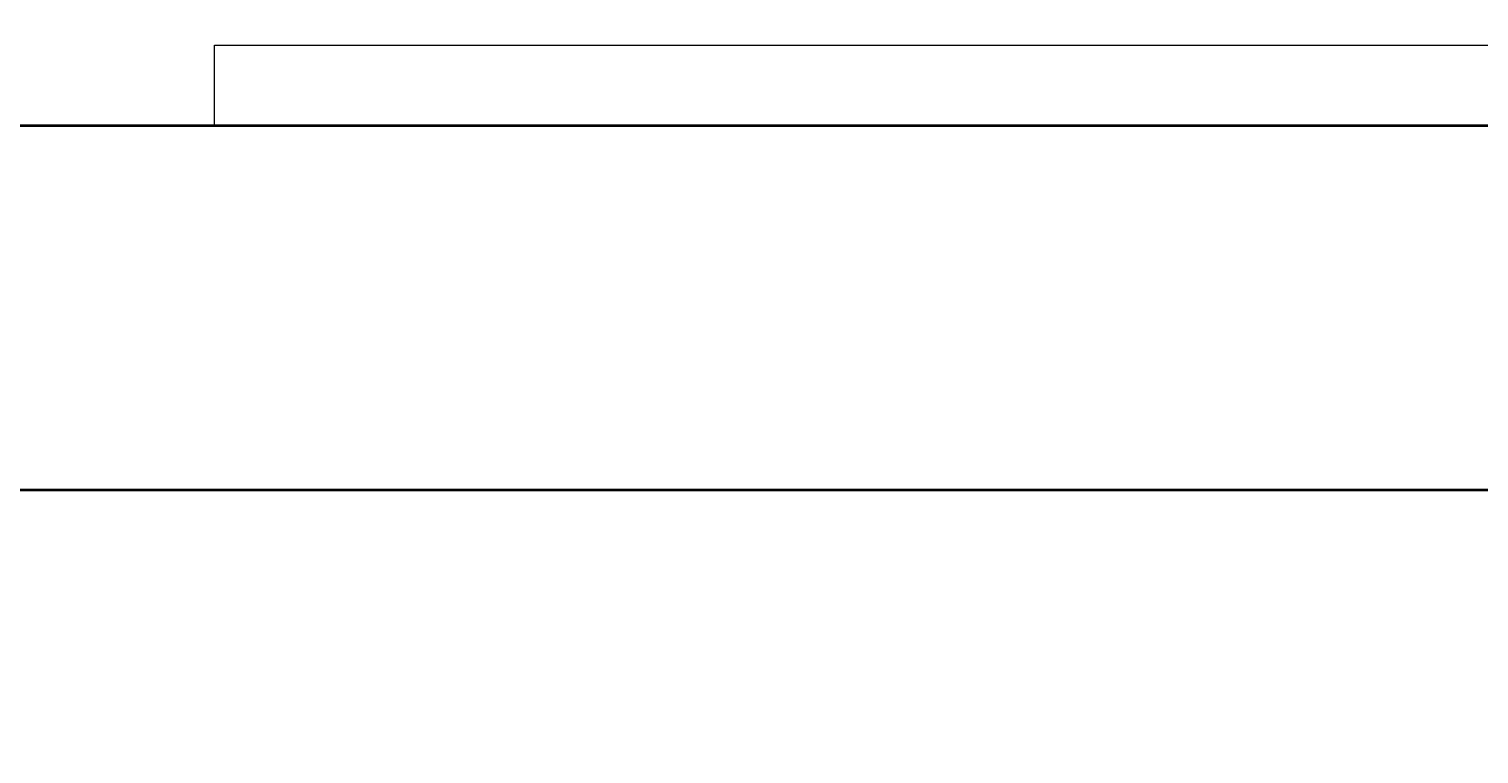
# Model space of a CAD drawing. Units: millimetres. Extents: x 27017497 to 27018854, y 7058029 to 7059154.
# Tile 67 of 91: x 27018355 to 27018390, y 7058126 to 7058144. Entities that reach past the tile are written whole.
import ezdxf

# ---------------------------------------------------------------- set-up
doc = ezdxf.new("R2010")
doc.units = ezdxf.units.MM
for name, color, linetype, lineweight in [('A-ANNO-DIMS', 2, 'Continuous', 18), ('A-FLOR-CASE-PATT', 44, 'Continuous', 13), ('A-FURN', 8, 'Continuous', 18), ('A-WALL', 7, 'Continuous', 35)]:
    doc.layers.add(name, color=color, linetype=linetype, lineweight=lineweight)
doc.styles.get("Standard").update_dxf_attribs({"font": 'arial.ttf'})
doc.dimstyles.get("Standard").update_dxf_attribs({"dimtxt": 0.18, "dimasz": 0.18, "dimexe": 0.18, "dimexo": 0.0625, "dimgap": 0.09, "dimtad": 0, "dimtih": 1, "dimtoh": 1, "dimdec": 4, "dimzin": 0, "dimdsep": 46, "dimtxsty": 'Standard', "dimcen": 0.09, "dimadec": 0, "dimazin": 0, "dimtfac": 1, "dimtdec": 4, "dimtofl": 0, "dimtmove": 0, "dimatfit": 3, "dimfxl": 1, "dimtolj": 1, "dimtzin": 0, "dimarcsym": 0})

# ---------------------------------------------------------------- blocks, each defined once
blk = doc.blocks.new('CAMMAT')
for p, q in [((1.27313, 0), (-1.27313, 0)), ((1.27313, 0), (1.27313, -0.05)), ((1.27313, -0.05), (-1.27313, -0.05))]:
    blk.add_line(p, q)
blk = doc.blocks.new('*D47')
at = {"layer": 'A-ANNO-DIMS', "color": 0, "lineweight": -2, "transparency": 16777216}
for p, q in [((27017561.166, 7058294.35), (27017561.166, 7058028.6)), ((27018790.606, 7058294.35), (27018790.606, 7058028.6)), ((27017561.346, 7058028.78), (27018175.431, 7058028.78)), ((27018790.426, 7058028.78), (27018176.341, 7058028.78))]:
    blk.add_line(p, q, dxfattribs=at)
at = {"layer": 'A-ANNO-DIMS', "color": 0, "transparency": 16777216}
for points in [[(27017561.346, 7058028.81), (27017561.346, 7058028.75), (27017561.166, 7058028.78)], [(27018790.426, 7058028.81), (27018790.426, 7058028.75), (27018790.606, 7058028.78)]]:
    blk.add_solid(points, dxfattribs=at)
at = {"layer": 'Defpoints', "color": 0, "transparency": 16777216}
for p in [(27017561.166, 7058294.412), (27018790.606, 7058294.412), (27018790.606, 7058028.78)]:
    blk.add_point(p, dxfattribs=at)
at = {"layer": 'A-ANNO-DIMS', "color": 0, "transparency": 16777216, "insert": (27018175.886, 7058028.78), "char_height": 0.18, "attachment_point": 5}
blk.add_mtext('\\A1;1229.4', dxfattribs=at)
blk = doc.blocks.new('*D48')
at = {"layer": 'A-ANNO-DIMS', "color": 0, "lineweight": -2, "transparency": 16777216}
for p, q in [((27018463.498, 7058622.912), (27017497.536, 7058622.912)), ((27017497.716, 7058622.732), (27017497.716, 7058357.753)), ((27017497.716, 7058092.41), (27017497.716, 7058357.389)), ((27018555.129, 7058092.23), (27017497.536, 7058092.23))]:
    blk.add_line(p, q, dxfattribs=at)
at = {"layer": 'A-ANNO-DIMS', "color": 0, "transparency": 16777216}
for points in [[(27017497.686, 7058622.732), (27017497.746, 7058622.732), (27017497.716, 7058622.912)], [(27017497.686, 7058092.41), (27017497.746, 7058092.41), (27017497.716, 7058092.23)]]:
    blk.add_solid(points, dxfattribs=at)
at = {"layer": 'Defpoints', "color": 0, "transparency": 16777216}
for p in [(27018463.561, 7058622.912), (27017497.716, 7058092.23), (27018555.192, 7058092.23)]:
    blk.add_point(p, dxfattribs=at)
at = {"layer": 'A-ANNO-DIMS', "color": 0, "transparency": 16777216, "insert": (27017497.716, 7058357.571), "char_height": 0.18, "attachment_point": 5}
blk.add_mtext('\\A1;530.7', dxfattribs=at)

msp = doc.modelspace()

# ---------------------------------------------------------------- hatches: boundary and pattern name
at = {"layer": 'A-FLOR-CASE-PATT'}
h = msp.add_hatch(color=256, dxfattribs=at)
h.dxf.hatch_style = 1
edge = h.paths.add_edge_path()
edge.add_line((27018341.343, 7058207.055), (27018330.837, 7058207.055))
edge.add_line((27018330.837, 7058207.055), (27018330.837, 7058203.02))
edge.add_line((27018330.837, 7058203.02), (27018338.424, 7058203.02))
edge.add_ellipse((27018338.23, 7058202.551), major_axis=(0.528, 0), ratio=0.888892, start_angle=0, end_angle=90, ccw=False)
edge.add_line((27018338.758, 7058202.551), (27018338.758, 7058202.238))
edge.add_line((27018338.758, 7058202.238), (27018330.837, 7058201.488))
edge.add_line((27018330.837, 7058201.488), (27018330.837, 7058199.747))
edge.add_line((27018330.837, 7058199.747), (27018338.424, 7058199.747))
edge.add_ellipse((27018338.23, 7058199.277), major_axis=(0.528, 0), ratio=0.888892, start_angle=0, end_angle=90, ccw=False)
edge.add_line((27018338.758, 7058199.277), (27018338.758, 7058198.964))
edge.add_line((27018338.758, 7058198.964), (27018330.837, 7058198.215))
edge.add_line((27018330.837, 7058198.215), (27018330.837, 7058193.415))
edge.add_line((27018330.837, 7058193.415), (27018338.284, 7058190.704))
edge.add_ellipse((27018337.942, 7058190.329), major_axis=(0.496, -0.181), ratio=0.888892, start_angle=0, end_angle=90, ccw=False)
edge.add_line((27018338.439, 7058190.148), (27018338.331, 7058189.854))
edge.add_line((27018338.331, 7058189.854), (27018330.837, 7058191.806))
edge.add_line((27018330.837, 7058191.806), (27018330.837, 7058188.22))
edge.add_line((27018330.837, 7058188.22), (27018338.424, 7058188.22))
edge.add_ellipse((27018338.23, 7058187.75), major_axis=(0.528, 0), ratio=0.888892, start_angle=0, end_angle=90, ccw=False)
edge.add_line((27018338.758, 7058187.75), (27018338.758, 7058187.437))
edge.add_line((27018338.758, 7058187.437), (27018330.837, 7058186.688))
edge.add_line((27018330.837, 7058186.688), (27018330.837, 7058181.982))
edge.add_line((27018330.837, 7058181.982), (27018338.424, 7058181.982))
edge.add_ellipse((27018338.23, 7058181.513), major_axis=(0.528, 0), ratio=0.888892, start_angle=0, end_angle=90, ccw=False)
edge.add_line((27018338.758, 7058181.513), (27018338.758, 7058181.199))
edge.add_line((27018338.758, 7058181.199), (27018330.837, 7058180.45))
edge.add_line((27018330.837, 7058180.45), (27018330.837, 7058178.709))
edge.add_line((27018330.837, 7058178.709), (27018338.424, 7058178.709))
edge.add_ellipse((27018338.23, 7058178.239), major_axis=(0.528, 0), ratio=0.888892, start_angle=0, end_angle=90, ccw=False)
edge.add_line((27018338.758, 7058178.239), (27018338.758, 7058177.926))
edge.add_line((27018338.758, 7058177.926), (27018330.837, 7058177.177))
edge.add_line((27018330.837, 7058177.177), (27018330.837, 7058173.878))
edge.add_line((27018330.837, 7058173.878), (27018338.284, 7058171.167))
edge.add_ellipse((27018337.942, 7058170.792), major_axis=(0.496, -0.181), ratio=0.888892, start_angle=0, end_angle=90, ccw=False)
edge.add_line((27018338.439, 7058170.611), (27018338.331, 7058170.317))
edge.add_line((27018338.331, 7058170.317), (27018330.837, 7058172.269))
edge.add_line((27018330.837, 7058172.269), (27018330.837, 7058168.293))
edge.add_line((27018330.837, 7058168.293), (27018338.424, 7058168.293))
edge.add_ellipse((27018338.23, 7058167.824), major_axis=(0.528, 0), ratio=0.888892, start_angle=0, end_angle=90, ccw=False)
edge.add_line((27018338.758, 7058167.824), (27018338.758, 7058167.511))
edge.add_line((27018338.758, 7058167.511), (27018330.837, 7058166.762))
edge.add_line((27018330.837, 7058166.762), (27018330.837, 7058160.389))
edge.add_line((27018330.837, 7058160.389), (27018338.424, 7058160.389))
edge.add_ellipse((27018338.23, 7058159.92), major_axis=(0.528, 0), ratio=0.888892, start_angle=0, end_angle=90, ccw=False)
edge.add_line((27018338.758, 7058159.92), (27018338.758, 7058159.607))
edge.add_line((27018338.758, 7058159.607), (27018330.837, 7058158.858))
edge.add_line((27018330.837, 7058158.858), (27018330.837, 7058157.116))
edge.add_line((27018330.837, 7058157.116), (27018338.424, 7058157.116))
edge.add_ellipse((27018338.23, 7058156.647), major_axis=(0.528, 0), ratio=0.888892, start_angle=0, end_angle=90, ccw=False)
edge.add_line((27018338.758, 7058156.647), (27018338.758, 7058156.334))
edge.add_line((27018338.758, 7058156.334), (27018330.837, 7058155.585))
edge.add_line((27018330.837, 7058155.585), (27018330.837, 7058150.784))
edge.add_line((27018330.837, 7058150.784), (27018338.284, 7058148.073))
edge.add_ellipse((27018337.942, 7058147.698), major_axis=(0.496, -0.181), ratio=0.888892, start_angle=0, end_angle=90, ccw=False)
edge.add_line((27018338.439, 7058147.517), (27018338.331, 7058147.223))
edge.add_line((27018338.331, 7058147.223), (27018330.837, 7058149.175))
edge.add_line((27018330.837, 7058149.175), (27018330.837, 7058145.589))
edge.add_line((27018330.837, 7058145.589), (27018338.424, 7058145.589))
edge.add_ellipse((27018338.23, 7058145.119), major_axis=(0.528, 0), ratio=0.888892, start_angle=0, end_angle=90, ccw=False)
edge.add_line((27018338.758, 7058145.119), (27018338.758, 7058144.806))
edge.add_line((27018338.758, 7058144.806), (27018330.837, 7058144.057))
edge.add_line((27018330.837, 7058144.057), (27018330.837, 7058141.912))
edge.add_line((27018330.837, 7058141.912), (27018341.343, 7058141.912))
edge.add_line((27018341.343, 7058141.912), (27018341.343, 7058207.055))
edge = h.paths.add_edge_path()
edge.add_line((27018330.112, 7058207.055), (27018319.606, 7058207.055))
edge.add_line((27018319.606, 7058207.055), (27018319.606, 7058141.912))
edge.add_line((27018319.606, 7058141.912), (27018330.112, 7058141.912))
edge.add_line((27018330.112, 7058141.912), (27018330.112, 7058144.024))
edge.add_line((27018330.112, 7058144.024), (27018322.543, 7058144.024))
edge.add_ellipse((27018322.736, 7058144.493), major_axis=(0.528, 0), ratio=0.888892, start_angle=180, end_angle=270, ccw=False)
edge.add_line((27018322.208, 7058144.493), (27018322.208, 7058145.291))
edge.add_ellipse((27018322.736, 7058145.119), major_axis=(0.528, 0), ratio=0.888892, start_angle=90, end_angle=180, ccw=False)
edge.add_line((27018322.736, 7058145.589), (27018330.112, 7058145.589))
edge.add_line((27018330.112, 7058145.589), (27018330.112, 7058149.382))
edge.add_line((27018330.112, 7058149.382), (27018322.826, 7058152.034))
edge.add_ellipse((27018323.168, 7058152.409), major_axis=(0.496, -0.181), ratio=0.888892, start_angle=180, end_angle=270, ccw=False)
edge.add_line((27018322.672, 7058152.59), (27018322.945, 7058153.34))
edge.add_ellipse((27018323.382, 7058152.997), major_axis=(0.496, -0.181), ratio=0.888892, start_angle=90, end_angle=180, ccw=False)
edge.add_line((27018323.543, 7058153.439), (27018330.112, 7058151.048))
edge.add_line((27018330.112, 7058151.048), (27018330.112, 7058155.551))
edge.add_line((27018330.112, 7058155.551), (27018322.543, 7058155.551))
edge.add_ellipse((27018322.736, 7058156.021), major_axis=(0.528, 0), ratio=0.888892, start_angle=180, end_angle=270, ccw=False)
edge.add_line((27018322.208, 7058156.021), (27018322.208, 7058156.819))
edge.add_ellipse((27018322.736, 7058156.647), major_axis=(0.528, 0), ratio=0.888892, start_angle=90, end_angle=180, ccw=False)
edge.add_line((27018322.736, 7058157.116), (27018330.112, 7058157.116))
edge.add_line((27018330.112, 7058157.116), (27018330.112, 7058158.824))
edge.add_line((27018330.112, 7058158.824), (27018322.543, 7058158.824))
edge.add_ellipse((27018322.736, 7058159.294), major_axis=(0.528, 0), ratio=0.888892, start_angle=180, end_angle=270, ccw=False)
edge.add_line((27018322.208, 7058159.294), (27018322.208, 7058160.092))
edge.add_ellipse((27018322.736, 7058159.92), major_axis=(0.528, 0), ratio=0.888892, start_angle=90, end_angle=180, ccw=False)
edge.add_line((27018322.736, 7058160.389), (27018330.112, 7058160.389))
edge.add_line((27018330.112, 7058160.389), (27018330.112, 7058166.728))
edge.add_line((27018330.112, 7058166.728), (27018322.543, 7058166.728))
edge.add_ellipse((27018322.736, 7058167.198), major_axis=(0.528, 0), ratio=0.888892, start_angle=180, end_angle=270, ccw=False)
edge.add_line((27018322.208, 7058167.198), (27018322.208, 7058167.996))
edge.add_ellipse((27018322.736, 7058167.824), major_axis=(0.528, 0), ratio=0.888892, start_angle=90, end_angle=180, ccw=False)
edge.add_line((27018322.736, 7058168.293), (27018330.112, 7058168.293))
edge.add_line((27018330.112, 7058168.293), (27018330.112, 7058172.476))
edge.add_line((27018330.112, 7058172.476), (27018322.826, 7058175.128))
edge.add_ellipse((27018323.168, 7058175.503), major_axis=(0.496, -0.181), ratio=0.888892, start_angle=180, end_angle=270, ccw=False)
edge.add_line((27018322.672, 7058175.684), (27018322.945, 7058176.433))
edge.add_ellipse((27018323.382, 7058176.091), major_axis=(0.496, -0.181), ratio=0.888892, start_angle=90, end_angle=180, ccw=False)
edge.add_line((27018323.543, 7058176.533), (27018330.112, 7058174.142))
edge.add_line((27018330.112, 7058174.142), (27018330.112, 7058177.144))
edge.add_line((27018330.112, 7058177.144), (27018322.543, 7058177.144))
edge.add_ellipse((27018322.736, 7058177.613), major_axis=(0.528, 0), ratio=0.888892, start_angle=180, end_angle=270, ccw=False)
edge.add_line((27018322.208, 7058177.613), (27018322.208, 7058178.411))
edge.add_ellipse((27018322.736, 7058178.239), major_axis=(0.528, 0), ratio=0.888892, start_angle=90, end_angle=180, ccw=False)
edge.add_line((27018322.736, 7058178.709), (27018330.112, 7058178.709))
edge.add_line((27018330.112, 7058178.709), (27018330.112, 7058180.417))
edge.add_line((27018330.112, 7058180.417), (27018322.543, 7058180.417))
edge.add_ellipse((27018322.736, 7058180.886), major_axis=(0.528, 0), ratio=0.888892, start_angle=180, end_angle=270, ccw=False)
edge.add_line((27018322.208, 7058180.886), (27018322.208, 7058181.684))
edge.add_ellipse((27018322.736, 7058181.513), major_axis=(0.528, 0), ratio=0.888892, start_angle=90, end_angle=180, ccw=False)
edge.add_line((27018322.736, 7058181.982), (27018330.112, 7058181.982))
edge.add_line((27018330.112, 7058181.982), (27018330.112, 7058186.655))
edge.add_line((27018330.112, 7058186.655), (27018322.543, 7058186.655))
edge.add_ellipse((27018322.736, 7058187.124), major_axis=(0.528, 0), ratio=0.888892, start_angle=180, end_angle=270, ccw=False)
edge.add_line((27018322.208, 7058187.124), (27018322.208, 7058187.922))
edge.add_ellipse((27018322.736, 7058187.75), major_axis=(0.528, 0), ratio=0.888892, start_angle=90, end_angle=180, ccw=False)
edge.add_line((27018322.736, 7058188.22), (27018330.112, 7058188.22))
edge.add_line((27018330.112, 7058188.22), (27018330.112, 7058192.013))
edge.add_line((27018330.112, 7058192.013), (27018322.826, 7058194.665))
edge.add_ellipse((27018323.168, 7058195.04), major_axis=(0.496, -0.181), ratio=0.888892, start_angle=180, end_angle=270, ccw=False)
edge.add_line((27018322.672, 7058195.22), (27018322.945, 7058195.97))
edge.add_ellipse((27018323.382, 7058195.628), major_axis=(0.496, -0.181), ratio=0.888892, start_angle=90, end_angle=180, ccw=False)
edge.add_line((27018323.543, 7058196.069), (27018330.112, 7058193.678))
edge.add_line((27018330.112, 7058193.678), (27018330.112, 7058198.182))
edge.add_line((27018330.112, 7058198.182), (27018322.543, 7058198.182))
edge.add_ellipse((27018322.736, 7058198.651), major_axis=(0.528, 0), ratio=0.888892, start_angle=180, end_angle=270, ccw=False)
edge.add_line((27018322.208, 7058198.651), (27018322.208, 7058199.449))
edge.add_ellipse((27018322.736, 7058199.277), major_axis=(0.528, 0), ratio=0.888892, start_angle=90, end_angle=180, ccw=False)
edge.add_line((27018322.736, 7058199.747), (27018330.112, 7058199.747))
edge.add_line((27018330.112, 7058199.747), (27018330.112, 7058201.455))
edge.add_line((27018330.112, 7058201.455), (27018322.543, 7058201.455))
edge.add_ellipse((27018322.736, 7058201.924), major_axis=(0.528, 0), ratio=0.888892, start_angle=180, end_angle=270, ccw=False)
edge.add_line((27018322.208, 7058201.924), (27018322.208, 7058202.722))
edge.add_ellipse((27018322.736, 7058202.551), major_axis=(0.528, 0), ratio=0.888892, start_angle=90, end_angle=180, ccw=False)
edge.add_line((27018322.736, 7058203.02), (27018330.112, 7058203.02))
edge.add_line((27018330.112, 7058203.02), (27018330.112, 7058207.055))
h.paths.add_polyline_path([(27018341.31, 7058294.412), (27018319.606, 7058294.412), (27018319.606, 7058207.1), (27018341.31, 7058207.1)])
h.paths.add_polyline_path([(27018354.358, 7058255.592), (27018354.358, 7058256.057, -0.414214), (27018354.869, 7058256.569), (27018346.477, 7058256.569, -0.414214), (27018345.197, 7058257.848), (27018345.197, 7058259.128, -0.414214), (27018346.477, 7058260.407), (27018343.868, 7058260.407, 0.290979), (27018341.551, 7058258.934), (27018341.551, 7058242.534, 0.290979), (27018343.868, 7058241.06), (27018346.477, 7058241.06, -0.414214), (27018345.197, 7058242.34), (27018345.197, 7058243.619, -0.414214), (27018346.477, 7058244.899), (27018353.078, 7058244.899, 0.414214), (27018354.358, 7058246.178)])
h.paths.add_polyline_path([(27018356.917, 7058260.407), (27018346.477, 7058260.407, 0.414214), (27018345.197, 7058259.128), (27018345.197, 7058257.848, 0.414214), (27018346.477, 7058256.569), (27018355.637, 7058256.569), (27018355.637, 7058244.899), (27018346.477, 7058244.899, 0.414214), (27018345.197, 7058243.619), (27018345.197, 7058242.34, 0.414214), (27018346.477, 7058241.06), (27018356.917, 7058241.06, 0.414214), (27018359.476, 7058243.619), (27018359.476, 7058257.848, 0.414214)])
h.paths.add_polyline_path([(27018355.637, 7058252.362), (27018355.637, 7058256.057, 0.490314), (27018354.997, 7058256.553, 0.490314), (27018354.358, 7058256.057), (27018354.358, 7058255.592), (27018354.358, 7058245.411, 0.490314), (27018354.997, 7058244.915, 0.490314), (27018355.637, 7058245.411)], flags=17)

# ---------------------------------------------------------------- linework, layer by layer
at = {"layer": 'A-WALL'}
for p, q in [((27018468.106, 7058141.912), (27018319.606, 7058141.912)), ((27018468.106, 7058132.912), (27018310.606, 7058132.912))]:
    msp.add_line(p, q, dxfattribs=at)

# ---------------------------------------------------------------- block references
at = {"layer": 'A-FURN', "xscale": 39.82996475819422, "yscale": 39.82996475819422, "zscale": 39.82996475819422, "rotation": 180}
msp.add_blockref('CAMMAT', (27018409.97, 7058141.912), dxfattribs=at)

# ---------------------------------------------------------------- dimensions: what is measured, and where the dimension line sits
at = {"layer": 'A-ANNO-DIMS'}
dim = msp.add_linear_dim(base=(27017497.716, 7058092.23), p1=(27018463.561, 7058622.912), p2=(27018555.192, 7058092.23), angle=90, dimstyle='Standard', override={"dimdec": 1, "dimlfac": 1, "dimrnd": 0, "dimzin": 0, "dimdsep": 46, "dimlunit": 2}, dxfattribs=at)
dim.commit()
dim.dimension.update_dxf_attribs({"geometry": '*D48', "text_midpoint": (27017497.716, 7058357.571)})
dim = msp.add_linear_dim(base=(27018790.606, 7058028.78), p1=(27017561.166, 7058294.412), p2=(27018790.606, 7058294.412), dimstyle='Standard', override={"dimdec": 1, "dimlfac": 1, "dimrnd": 0, "dimzin": 0, "dimdsep": 46, "dimlunit": 2}, dxfattribs=at)
dim.commit()
dim.dimension.update_dxf_attribs({"geometry": '*D47', "text_midpoint": (27018175.886, 7058028.78)})

doc.saveas('drawing.dxf')
